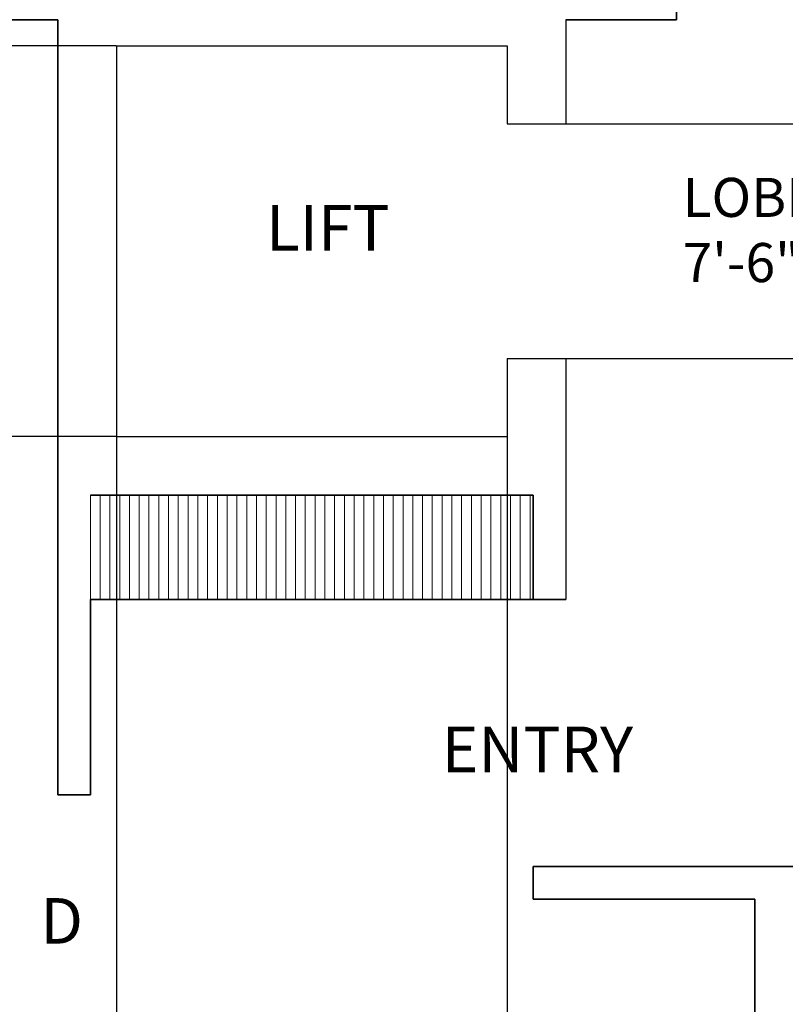
# Model space of a CAD drawing. Units: inches. Extents: x 3731 to 4318, y 1310 to 2388.
# Tile 30 of 57: x 3954 to 4072, y 1787 to 1938. Entities that reach past the tile are written whole.
import ezdxf

# ---------------------------------------------------------------- set-up
doc = ezdxf.new("R2010")
doc.units = ezdxf.units.IN
for name, color, linetype, lineweight in [('A-ANNO-DIMS', 2, 'Continuous', 18), ('A-ANNO-TEXT', 7, 'Continuous', 18), ('A-AREA-IDEN', 7, 'Continuous', 18), ('A-FLOR-EVTR', 4, 'Continuous', 25), ('A-FLOR-PATT', 252, 'Continuous', 13), ('A-WALL', 7, 'Continuous', 35)]:
    doc.layers.add(name, color=color, linetype=linetype, lineweight=lineweight)
doc.styles.get("Standard").update_dxf_attribs({"font": 'arial.ttf'})
doc.dimstyles.get("Standard").update_dxf_attribs({"dimtxt": 0.18, "dimasz": 0.18, "dimexe": 0.18, "dimexo": 0.0625, "dimgap": 0.09, "dimtad": 0, "dimtih": 1, "dimtoh": 1, "dimdec": 4, "dimzin": 0, "dimdsep": 46, "dimtxsty": 'Standard', "dimcen": 0.09, "dimadec": 0, "dimazin": 0, "dimtfac": 1, "dimtdec": 4, "dimtofl": 0, "dimtmove": 0, "dimatfit": 3, "dimfxl": 1, "dimtolj": 1, "dimtzin": 0, "dimarcsym": 0})

# ---------------------------------------------------------------- blocks, each defined once
blk = doc.blocks.new('*U8')
blk.add_line((0, 16), (0, 0))
blk = doc.blocks.new('*U9')
at = {"layer": 'A-FLOR-PATT', "color": 0, "linetype": 'ByBlock', "lineweight": -2, "transparency": 16777216}
for p in [(3965.21, 1849.38), (3966.71, 1849.38), (3968.21, 1849.38), (3969.71, 1849.38), (3971.21, 1849.38), (3972.71, 1849.38), (3974.21, 1849.38), (3975.71, 1849.38), (3977.21, 1849.38), (3978.71, 1849.38), (3980.21, 1849.38), (3981.71, 1849.38), (3983.21, 1849.38), (3984.71, 1849.38), (3986.21, 1849.38), (3987.71, 1849.38), (3989.21, 1849.38), (3990.71, 1849.38), (3992.21, 1849.38), (3993.71, 1849.38), (3995.21, 1849.38), (3996.71, 1849.38), (3998.21, 1849.38), (3999.71, 1849.38), (4001.21, 1849.38), (4002.71, 1849.38), (4004.21, 1849.38), (4005.71, 1849.38), (4007.21, 1849.38), (4008.71, 1849.38), (4010.21, 1849.38), (4011.71, 1849.38), (4013.21, 1849.38), (4014.71, 1849.38), (4016.21, 1849.38), (4017.71, 1849.38), (4019.21, 1849.38), (4020.71, 1849.38), (4022.21, 1849.38), (4023.71, 1849.38), (4025.21, 1849.38), (4026.71, 1849.38), (4028.21, 1849.38), (4029.71, 1849.38), (4031.21, 1849.38), (4032.71, 1849.38)]:
    blk.add_blockref('*U8', p, dxfattribs=at)
blk = doc.blocks.new('*D44')
at = {"layer": 'A-ANNO-DIMS', "color": 0, "lineweight": -2, "transparency": 16777216}
for p, q in [((3969.21, 1874.32), (3969.21, 1310.25)), ((4029.21, 1874.32), (4029.21, 1310.25)), ((3969.39, 1310.43), (3998.99, 1310.43)), ((4029.03, 1310.43), (3999.43, 1310.43))]:
    blk.add_line(p, q, dxfattribs=at)
at = {"layer": 'A-ANNO-DIMS', "color": 0, "transparency": 16777216}
for points in [[(3969.39, 1310.46), (3969.39, 1310.4), (3969.21, 1310.43)], [(4029.03, 1310.46), (4029.03, 1310.4), (4029.21, 1310.43)]]:
    blk.add_solid(points, dxfattribs=at)
at = {"layer": 'Defpoints', "color": 0, "transparency": 16777216}
for p in [(3969.21, 1874.38), (4029.21, 1874.38), (4029.21, 1310.43)]:
    blk.add_point(p, dxfattribs=at)
at = {"layer": 'A-ANNO-DIMS', "color": 0, "transparency": 16777216, "insert": (3999.21, 1310.43), "char_height": 0.18, "attachment_point": 5}
blk.add_mtext('\\A1;60', dxfattribs=at)
blk = doc.blocks.new('*D45')
at = {"layer": 'A-ANNO-DIMS', "color": 0, "lineweight": -2, "transparency": 16777216}
for p, q in [((3969.15, 1934.38), (3731.41, 1934.38)), ((3731.59, 1934.2), (3731.59, 1904.56)), ((3731.59, 1874.56), (3731.59, 1904.2)), ((3969.15, 1874.38), (3731.41, 1874.38))]:
    blk.add_line(p, q, dxfattribs=at)
at = {"layer": 'A-ANNO-DIMS', "color": 0, "transparency": 16777216}
for points in [[(3731.56, 1934.2), (3731.62, 1934.2), (3731.59, 1934.38)], [(3731.56, 1874.56), (3731.62, 1874.56), (3731.59, 1874.38)]]:
    blk.add_solid(points, dxfattribs=at)
at = {"layer": 'Defpoints', "color": 0, "transparency": 16777216}
for p in [(3731.59, 1934.38), (3969.21, 1934.38), (3969.21, 1874.38)]:
    blk.add_point(p, dxfattribs=at)
at = {"layer": 'A-ANNO-DIMS', "color": 0, "transparency": 16777216, "insert": (3731.59, 1904.38), "char_height": 0.18, "attachment_point": 5}
blk.add_mtext('\\A1;60', dxfattribs=at)
blk = doc.blocks.new('*D50')
at = {"layer": 'A-ANNO-DIMS', "color": 0, "lineweight": -2, "transparency": 16777216}
for p, q in [((4029.27, 1922.38), (4318.34, 1922.38)), ((4318.16, 1922.2), (4318.16, 1904.56)), ((4318.16, 1886.56), (4318.16, 1904.2)), ((4029.27, 1886.38), (4318.34, 1886.38))]:
    blk.add_line(p, q, dxfattribs=at)
at = {"layer": 'A-ANNO-DIMS', "color": 0, "transparency": 16777216}
for points in [[(4318.13, 1922.2), (4318.19, 1922.2), (4318.16, 1922.38)], [(4318.13, 1886.56), (4318.19, 1886.56), (4318.16, 1886.38)]]:
    blk.add_solid(points, dxfattribs=at)
at = {"layer": 'Defpoints', "color": 0, "transparency": 16777216}
for p in [(4029.21, 1922.38), (4318.16, 1922.38), (4029.21, 1886.38)]:
    blk.add_point(p, dxfattribs=at)
at = {"layer": 'A-ANNO-DIMS', "color": 0, "transparency": 16777216, "insert": (4318.16, 1904.38), "char_height": 0.18, "attachment_point": 5}
blk.add_mtext('\\A1;36', dxfattribs=at)

msp = doc.modelspace()

# ---------------------------------------------------------------- linework, layer by layer
at = {"layer": 'A-FLOR-EVTR'}
for p, q in [((4038.21, 1938.38), (4038.21, 1922.38)), ((3969.21, 1934.38), (4029.21, 1934.38)), ((3969.21, 1934.38), (3969.21, 1874.38)), ((4029.21, 1934.38), (4029.21, 1922.38)), ((4029.21, 1922.38), (4038.21, 1922.38)), ((4029.21, 1886.38), (4038.21, 1886.38)), ((4029.21, 1886.38), (4029.21, 1874.38)), ((4038.21, 1886.38), (4038.21, 1849.38)), ((3969.21, 1874.38), (4029.21, 1874.38))]:
    msp.add_line(p, q, dxfattribs=at)
at = {"layer": 'A-WALL'}
for p, q in [((4055.21, 1938.38), (4055.21, 1943.38)), ((3840.21, 1938.38), (3960.21, 1938.38)), ((3960.21, 1938.38), (3960.21, 1819.38)), ((4038.21, 1938.38), (4055.21, 1938.38)), ((3965.21, 1865.38), (4033.21, 1865.38)), ((4033.21, 1865.38), (4033.21, 1849.38)), ((4033.21, 1849.38), (3965.21, 1849.38)), ((3965.21, 1849.38), (3965.21, 1819.38)), ((4033.21, 1849.38), (4038.21, 1849.38)), ((3960.21, 1819.38), (3965.21, 1819.38)), ((4033.21, 1808.38), (4108.21, 1808.38)), ((4033.21, 1808.38), (4033.21, 1803.38)), ((4033.21, 1803.38), (4067.21, 1803.38)), ((4067.21, 1803.38), (4067.21, 1554.38))]:
    msp.add_line(p, q, dxfattribs=at)

# ---------------------------------------------------------------- block references
at = {"layer": 'A-FLOR-PATT'}
msp.add_blockref('*U9', (0, 0), dxfattribs=at)

# ---------------------------------------------------------------- texts
at = {"layer": 'A-ANNO-TEXT', "char_height": 7, "attachment_point": 1}
for s, insert in [('ENTRY', (4019.15, 1829.85)), ('D', (3957.51, 1803.53))]:
    msp.add_mtext_dynamic_manual_height_columns(s, width=10.4564, gutter_width=12.5, heights=[0], dxfattribs=dict(at, insert=insert))
at = {"layer": 'A-AREA-IDEN', "attachment_point": 1}
for s, insert, char_height in [('LOBBY\\P7\'-6"X7\'-0"', (4056.14, 1914.1), 6), ('LIFT', (3992.18, 1909.91), 7)]:
    msp.add_mtext_dynamic_manual_height_columns(s, width=47.0437, gutter_width=12.5, heights=[0], dxfattribs=dict(at, insert=insert, char_height=char_height))

# ---------------------------------------------------------------- dimensions: what is measured, and where the dimension line sits
at = {"layer": 'A-ANNO-DIMS'}
for base, p1, p2, picture, middle in [((3731.59, 1934.38), (3969.21, 1874.38), (3969.21, 1934.38), '*D45', (3731.59, 1904.38)), ((4318.16, 1922.38), (4029.21, 1886.38), (4029.21, 1922.38), '*D50', (4318.16, 1904.38))]:
    dim = msp.add_linear_dim(base=base, p1=p1, p2=p2, angle=90, dimstyle='Standard', override={"dimdec": 0, "dimlfac": 1, "dimrnd": 0, "dimzin": 0, "dimdsep": 46, "dimlunit": 2}, dxfattribs=at)
    dim.commit()
    dim.dimension.update_dxf_attribs({"geometry": picture, "text_midpoint": middle})
dim = msp.add_linear_dim(base=(4029.21, 1310.43), p1=(3969.21, 1874.38), p2=(4029.21, 1874.38), dimstyle='Standard', override={"dimdec": 0, "dimlfac": 1, "dimrnd": 0, "dimzin": 0, "dimdsep": 46, "dimlunit": 2}, dxfattribs=at)
dim.commit()
dim.dimension.update_dxf_attribs({"geometry": '*D44', "text_midpoint": (3999.21, 1310.43)})

doc.saveas('drawing.dxf')
